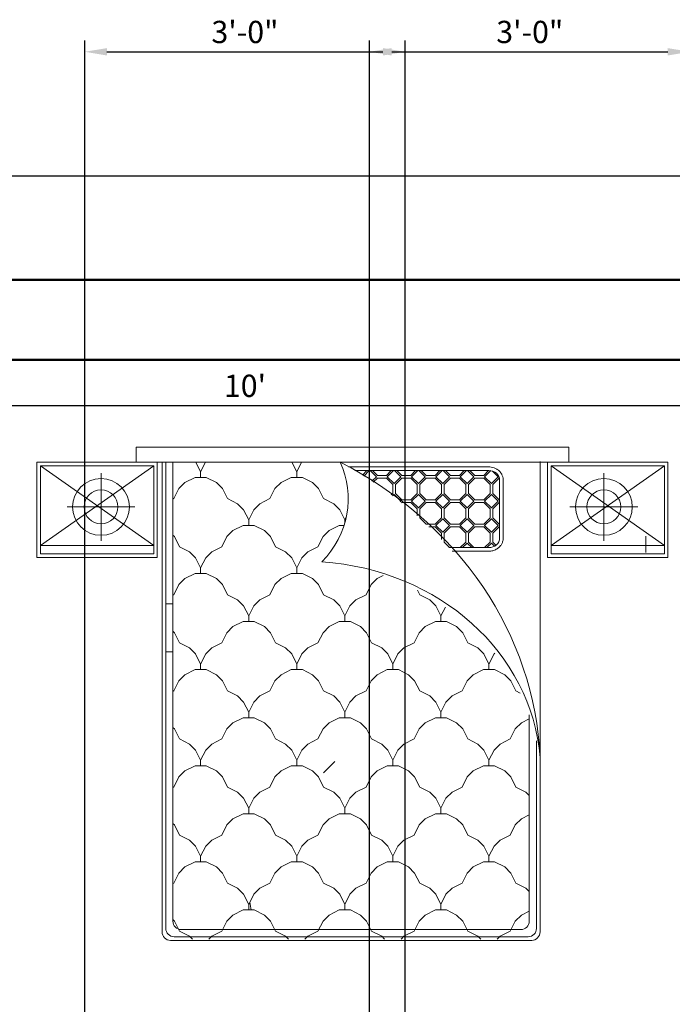
# Model space of a CAD drawing. Units: inches. Extents: x 2385 to 2740, y 1752 to 2305.
# Tile 14 of 15: x 2618 to 2691, y 2195 to 2305. Entities that reach past the tile are written whole.
import ezdxf

# ---------------------------------------------------------------- set-up
doc = ezdxf.new("R2010")
doc.units = ezdxf.units.IN
for name, color, linetype, lineweight in [('A-ANNO-DIMS', 2, 'Continuous', 18), ('A-FURN', 9, 'Continuous', 18), ('A-WALL', 7, 'Continuous', 50)]:
    doc.layers.add(name, color=color, linetype=linetype, lineweight=lineweight)
doc.styles.get("Standard").update_dxf_attribs({"font": 'arial.ttf'})
doc.dimstyles.new('Copy of ISO-25', dxfattribs={"dimtxt": 2.5, "dimasz": 2.5, "dimexe": 1.25, "dimexo": 0.625, "dimtad": 1, "dimdec": 1, "dimlunit": 4, "dimtxsty": 'Standard', "dimcen": 2.5, "dimadec": 0, "dimazin": 0, "dimtfac": 1, "dimtdec": 1, "dimtmove": 0, "dimatfit": 3, "dimfxl": 1, "dimarcsym": 0})

# ---------------------------------------------------------------- blocks, each defined once
blk = doc.blocks.new('A$C029D5C69')
for p, q in [((0.4164, 2.0693), (0.4164, 2.0066)), ((2.2315, 2.0693), (0.4164, 2.0693)), ((2.2315, 2.0066), (2.2315, 2.0693)), ((0, 1.606), (0, 2.0066)), ((0, 2.0066), (0.505, 2.0066)), ((0.0151, 1.6211), (0.0151, 1.9915)), ((0.0151, 1.9915), (0.4899, 1.9915)), ((0.4164, 2.0066), (2.2315, 2.0066)), ((0.4899, 1.9915), (0.4899, 1.6211)), ((0.505, 2.0066), (0.505, 1.606)), ((0.5252, 0.0351), (0.5252, 2.0066)), ((0.5403, 0.0502), (0.5403, 2.0066)), ((0.5706, 0.0805), (0.5706, 2.0066)), ((0.6869, 1.966), (0.6666, 2.0066)), ((0.7072, 2.0066), (0.6869, 1.966)), ((1.0902, 1.966), (1.0699, 2.0066)), ((1.1106, 2.0066), (1.0902, 1.966)), ((1.8954, 1.9865), (1.3081, 1.9865)), ((2.1114, 2.0087), (2.1114, 0.0351)), ((2.6479, 2.0066), (2.1429, 2.0066)), ((2.1429, 2.0066), (2.1429, 1.606)), ((2.6328, 1.9915), (2.158, 1.9915)), ((2.158, 1.9915), (2.158, 1.6211)), ((2.6328, 1.6211), (2.6328, 1.9915)), ((2.6479, 1.606), (2.6479, 2.0066)), ((0.2689, 1.9609), (0.2689, 1.6764)), ((0.6634, 1.9425), (0.621, 1.9213)), ((0.6634, 1.9425), (0.621, 1.9213)), ((0.6869, 1.9425), (0.6634, 1.9425)), ((0.6869, 1.9425), (0.6869, 1.966)), ((0.6869, 1.9425), (0.6869, 1.966)), ((0.6869, 1.9425), (0.7104, 1.9425)), ((0.7528, 1.9213), (0.7104, 1.9425)), ((0.7528, 1.9213), (0.7104, 1.9425)), ((1.0668, 1.9425), (1.0244, 1.9213)), ((1.0668, 1.9425), (1.0244, 1.9213)), ((1.0902, 1.9425), (1.0668, 1.9425)), ((1.0902, 1.9425), (1.0902, 1.966)), ((1.0902, 1.9425), (1.0902, 1.966)), ((1.0902, 1.9425), (1.1137, 1.9425)), ((1.1561, 1.9213), (1.1137, 1.9425)), ((1.1561, 1.9213), (1.1137, 1.9425)), ((1.8954, 1.9713), (1.3339, 1.9713)), ((1.3849, 1.9713), (1.3656, 1.952)), ((1.3945, 1.9713), (1.3714, 1.9483)), ((1.4249, 1.945), (1.3986, 1.9713)), ((1.4249, 1.945), (1.4059, 1.926)), ((1.4288, 1.9507), (1.4081, 1.9713)), ((1.4476, 1.9507), (1.4288, 1.9507)), ((1.4476, 1.9507), (1.4664, 1.9507)), ((1.487, 1.9713), (1.4664, 1.9507)), ((1.4966, 1.9713), (1.4703, 1.945)), ((1.4986, 1.9167), (1.4703, 1.945)), ((1.527, 1.945), (1.4986, 1.9167)), ((1.527, 1.945), (1.5007, 1.9713)), ((1.5309, 1.9507), (1.5102, 1.9713)), ((1.5497, 1.9507), (1.5309, 1.9507)), ((1.5497, 1.9507), (1.5685, 1.9507)), ((1.5891, 1.9713), (1.5685, 1.9507)), ((1.5987, 1.9713), (1.5724, 1.945)), ((1.6007, 1.9167), (1.5724, 1.945)), ((1.6291, 1.945), (1.6007, 1.9167)), ((1.6291, 1.945), (1.6028, 1.9713)), ((1.633, 1.9507), (1.6123, 1.9713)), ((1.6518, 1.9507), (1.633, 1.9507)), ((1.6518, 1.9507), (1.6706, 1.9507)), ((1.6912, 1.9713), (1.6706, 1.9507)), ((1.7008, 1.9713), (1.6745, 1.945)), ((1.7028, 1.9167), (1.6745, 1.945)), ((1.7312, 1.945), (1.7028, 1.9167)), ((1.7312, 1.945), (1.7049, 1.9713)), ((1.7351, 1.9507), (1.7144, 1.9713)), ((1.7539, 1.9507), (1.7351, 1.9507)), ((1.7539, 1.9507), (1.7727, 1.9507)), ((1.7933, 1.9713), (1.7727, 1.9507)), ((1.8029, 1.9713), (1.7766, 1.945)), ((1.8049, 1.9167), (1.7766, 1.945)), ((1.8333, 1.945), (1.8049, 1.9167)), ((1.8333, 1.945), (1.807, 1.9713)), ((1.8372, 1.9507), (1.8165, 1.9713)), ((1.856, 1.9507), (1.8372, 1.9507)), ((1.856, 1.9507), (1.8748, 1.9507)), ((1.8954, 1.9713), (1.8748, 1.9507)), ((1.9043, 1.9707), (1.8787, 1.945)), ((1.907, 1.9167), (1.8787, 1.945)), ((1.9354, 1.945), (1.907, 1.9167)), ((1.9354, 1.945), (1.9114, 1.969)), ((2.379, 1.9609), (2.379, 1.6764)), ((0.621, 1.9213), (0.5955, 1.8958)), ((0.7783, 1.8958), (0.7528, 1.9213)), ((1.0243, 1.9213), (0.9988, 1.8958)), ((1.1816, 1.8958), (1.1561, 1.9213)), ((1.4288, 1.9394), (1.4116, 1.9222)), ((1.4288, 1.9393), (1.4476, 1.9393)), ((1.4664, 1.9393), (1.4476, 1.9393)), ((1.493, 1.9128), (1.4664, 1.9394)), ((1.493, 1.8752), (1.493, 1.9128)), ((1.5309, 1.9394), (1.5043, 1.9128)), ((1.5043, 1.8752), (1.5043, 1.9128)), ((1.5309, 1.9393), (1.5497, 1.9393)), ((1.5685, 1.9393), (1.5497, 1.9393)), ((1.595, 1.9128), (1.5685, 1.9394)), ((1.595, 1.8752), (1.595, 1.9128)), ((1.633, 1.9394), (1.6064, 1.9128)), ((1.6064, 1.8752), (1.6064, 1.9128)), ((1.633, 1.9393), (1.6518, 1.9393)), ((1.6706, 1.9393), (1.6518, 1.9393)), ((1.6971, 1.9128), (1.6706, 1.9394)), ((1.6971, 1.8752), (1.6971, 1.9128)), ((1.7351, 1.9394), (1.7085, 1.9128)), ((1.7085, 1.8752), (1.7085, 1.9128)), ((1.7351, 1.9393), (1.7539, 1.9393)), ((1.7727, 1.9393), (1.7539, 1.9393)), ((1.7992, 1.9128), (1.7727, 1.9394)), ((1.7992, 1.8752), (1.7992, 1.9128)), ((1.8372, 1.9394), (1.8106, 1.9128)), ((1.8106, 1.8752), (1.8106, 1.9128)), ((1.8372, 1.9393), (1.856, 1.9393)), ((1.8748, 1.9393), (1.856, 1.9393)), ((1.9013, 1.9128), (1.8748, 1.9394)), ((1.9013, 1.8752), (1.9013, 1.9128)), ((1.9393, 1.9394), (1.9127, 1.9128)), ((1.9127, 1.8752), (1.9127, 1.9128)), ((1.9393, 1.9393), (1.9404, 1.9393)), ((1.9414, 1.688), (1.9414, 1.931)), ((1.9565, 1.688), (1.9565, 1.931)), ((0.5955, 1.8958), (0.5743, 1.8534)), ((0.7995, 1.8534), (0.7783, 1.8958)), ((0.9989, 1.8958), (0.9777, 1.8534)), ((1.2028, 1.8534), (1.1816, 1.8958)), ((1.493, 1.8752), (1.4867, 1.869)), ((1.4986, 1.8713), (1.4922, 1.8648)), ((1.527, 1.8429), (1.4986, 1.8713)), ((1.5309, 1.8486), (1.5043, 1.8752)), ((1.595, 1.8752), (1.5685, 1.8486)), ((1.6007, 1.8713), (1.5724, 1.8429)), ((1.6291, 1.8429), (1.6007, 1.8713)), ((1.633, 1.8486), (1.6064, 1.8752)), ((1.6971, 1.8752), (1.6706, 1.8486)), ((1.7028, 1.8713), (1.6745, 1.8429)), ((1.7312, 1.8429), (1.7028, 1.8713)), ((1.7351, 1.8486), (1.7085, 1.8752)), ((1.7992, 1.8752), (1.7727, 1.8486)), ((1.8049, 1.8713), (1.7766, 1.8429)), ((1.8333, 1.8429), (1.8049, 1.8713)), ((1.8372, 1.8486), (1.8106, 1.8752)), ((1.9013, 1.8752), (1.8748, 1.8486)), ((1.907, 1.8713), (1.8787, 1.8429)), ((1.9354, 1.8429), (1.907, 1.8713)), ((1.9393, 1.8486), (1.9127, 1.8752)), ((0.1267, 1.8186), (0.4111, 1.8186)), ((0.5743, 1.8534), (0.5706, 1.8515)), ((0.5743, 1.8534), (0.5706, 1.8515)), ((0.8419, 1.8322), (0.7995, 1.8534)), ((0.8419, 1.8322), (0.7995, 1.8534)), ((0.8674, 1.8067), (0.8419, 1.8322)), ((0.9352, 1.8322), (0.9097, 1.8067)), ((0.9777, 1.8534), (0.9353, 1.8322)), ((0.9777, 1.8534), (0.9353, 1.8322)), ((1.2452, 1.8322), (1.2028, 1.8534)), ((1.2452, 1.8322), (1.2028, 1.8534)), ((1.2707, 1.8067), (1.2452, 1.8322)), ((1.527, 1.8429), (1.5242, 1.8401)), ((1.5309, 1.8373), (1.5295, 1.8359)), ((1.5497, 1.8486), (1.5309, 1.8486)), ((1.5309, 1.8373), (1.5497, 1.8373)), ((1.5497, 1.8486), (1.5685, 1.8486)), ((1.5685, 1.8373), (1.5497, 1.8373)), ((1.595, 1.8107), (1.5685, 1.8373)), ((1.6007, 1.8146), (1.5724, 1.8429)), ((1.6291, 1.8429), (1.6007, 1.8146)), ((1.633, 1.8373), (1.6064, 1.8107)), ((1.6518, 1.8486), (1.633, 1.8486)), ((1.633, 1.8373), (1.6518, 1.8373)), ((1.6518, 1.8486), (1.6706, 1.8486)), ((1.6706, 1.8373), (1.6518, 1.8373)), ((1.6971, 1.8107), (1.6706, 1.8373)), ((1.7028, 1.8146), (1.6745, 1.8429)), ((1.7312, 1.8429), (1.7028, 1.8146)), ((1.7351, 1.8373), (1.7085, 1.8107)), ((1.7539, 1.8486), (1.7351, 1.8486)), ((1.7351, 1.8373), (1.7539, 1.8373)), ((1.7539, 1.8486), (1.7727, 1.8486)), ((1.7727, 1.8373), (1.7539, 1.8373)), ((1.7992, 1.8107), (1.7727, 1.8373)), ((1.8049, 1.8146), (1.7766, 1.8429)), ((1.8333, 1.8429), (1.8049, 1.8146)), ((1.8372, 1.8373), (1.8106, 1.8107)), ((1.856, 1.8486), (1.8372, 1.8486)), ((1.8372, 1.8373), (1.856, 1.8373)), ((1.856, 1.8486), (1.8748, 1.8486)), ((1.8748, 1.8373), (1.856, 1.8373)), ((1.9013, 1.8107), (1.8748, 1.8373)), ((1.907, 1.8146), (1.8787, 1.8429)), ((1.9354, 1.8429), (1.907, 1.8146)), ((1.9393, 1.8373), (1.9127, 1.8107)), ((1.9414, 1.8486), (1.9393, 1.8486)), ((1.9393, 1.8373), (1.9414, 1.8373)), ((2.2367, 1.8186), (2.5212, 1.8186)), ((0.8886, 1.7643), (0.8674, 1.8067)), ((0.9098, 1.8067), (0.8886, 1.7643)), ((1.2919, 1.7643), (1.2707, 1.8067)), ((1.2981, 1.7768), (1.2919, 1.7643)), ((1.595, 1.7806), (1.595, 1.8107)), ((1.6064, 1.7731), (1.6064, 1.8107)), ((1.6971, 1.7731), (1.6971, 1.8107)), ((1.7085, 1.7731), (1.7085, 1.8107)), ((1.7992, 1.7731), (1.7992, 1.8107)), ((1.8106, 1.7731), (1.8106, 1.8107)), ((1.9013, 1.7731), (1.9013, 1.8107)), ((1.9127, 1.7731), (1.9127, 1.8107)), ((0.8651, 1.7408), (0.8227, 1.7196)), ((0.8651, 1.7408), (0.8227, 1.7196)), ((0.912, 1.7408), (0.8651, 1.7408)), ((0.8886, 1.7408), (0.8886, 1.7643)), ((0.9544, 1.7196), (0.912, 1.7408)), ((0.9544, 1.7196), (0.912, 1.7408)), ((1.2684, 1.7408), (1.226, 1.7196)), ((1.2684, 1.7408), (1.226, 1.7196)), ((1.2885, 1.7408), (1.2684, 1.7408)), ((1.2919, 1.7519), (1.2919, 1.7643)), ((1.633, 1.7465), (1.6064, 1.7731)), ((1.6518, 1.7465), (1.633, 1.7465)), ((1.6443, 1.7352), (1.6518, 1.7352)), ((1.6518, 1.7465), (1.6706, 1.7465)), ((1.6706, 1.7352), (1.6518, 1.7352)), ((1.6971, 1.7731), (1.6706, 1.7465)), ((1.6971, 1.7086), (1.6706, 1.7352)), ((1.7028, 1.7692), (1.6745, 1.7408)), ((1.7028, 1.7125), (1.6745, 1.7408)), ((1.7312, 1.7408), (1.7028, 1.7692)), ((1.7312, 1.7408), (1.7028, 1.7125)), ((1.7351, 1.7465), (1.7085, 1.7731)), ((1.7351, 1.7352), (1.7085, 1.7086)), ((1.7539, 1.7465), (1.7351, 1.7465)), ((1.7351, 1.7352), (1.7539, 1.7352)), ((1.7539, 1.7465), (1.7727, 1.7465)), ((1.7727, 1.7352), (1.7539, 1.7352)), ((1.7992, 1.7731), (1.7727, 1.7465)), ((1.7992, 1.7086), (1.7727, 1.7352)), ((1.8049, 1.7692), (1.7766, 1.7408)), ((1.8049, 1.7125), (1.7766, 1.7408)), ((1.8333, 1.7408), (1.8049, 1.7692)), ((1.8333, 1.7408), (1.8049, 1.7125)), ((1.8372, 1.7465), (1.8106, 1.7731)), ((1.8372, 1.7352), (1.8106, 1.7086)), ((1.856, 1.7465), (1.8372, 1.7465)), ((1.8372, 1.7352), (1.856, 1.7352)), ((1.856, 1.7465), (1.8748, 1.7465)), ((1.8748, 1.7352), (1.856, 1.7352)), ((1.9013, 1.7731), (1.8748, 1.7465)), ((1.9013, 1.7086), (1.8748, 1.7352)), ((1.907, 1.7692), (1.8787, 1.7408)), ((1.907, 1.7125), (1.8787, 1.7408)), ((1.9354, 1.7408), (1.907, 1.7692)), ((1.9354, 1.7408), (1.907, 1.7125)), ((1.9393, 1.7465), (1.9127, 1.7731)), ((1.9393, 1.7352), (1.9127, 1.7086)), ((1.9414, 1.7465), (1.9393, 1.7465)), ((1.9393, 1.7352), (1.9414, 1.7352)), ((0.5766, 1.6941), (0.5706, 1.7002)), ((0.5978, 1.6517), (0.5766, 1.6941)), ((0.7972, 1.6941), (0.776, 1.6517)), ((0.8227, 1.7196), (0.7972, 1.6941)), ((0.98, 1.6941), (0.9545, 1.7196)), ((1.0011, 1.6517), (0.9799, 1.6941)), ((1.2005, 1.6941), (1.1793, 1.6517)), ((1.226, 1.7196), (1.2005, 1.6941)), ((1.6971, 1.682), (1.6971, 1.7086)), ((1.7085, 1.671), (1.7085, 1.7086)), ((1.7992, 1.671), (1.7992, 1.7086)), ((1.8106, 1.671), (1.8106, 1.7086)), ((1.9013, 1.671), (1.9013, 1.7086)), ((1.9127, 1.671), (1.9127, 1.7086)), ((2.5551, 1.6275), (2.5551, 1.696)), ((1.7318, 1.6477), (1.7085, 1.671)), ((1.7992, 1.671), (1.7759, 1.6477)), ((1.8049, 1.6671), (1.7855, 1.6477)), ((1.8244, 1.6477), (1.8049, 1.6671)), ((1.8339, 1.6477), (1.8106, 1.671)), ((1.9013, 1.671), (1.878, 1.6477)), ((1.907, 1.6671), (1.8876, 1.6477)), ((1.9202, 1.6539), (1.907, 1.6671)), ((1.926, 1.6577), (1.9127, 1.671)), ((0.4899, 1.6211), (0.0151, 1.6211)), ((0.6402, 1.6305), (0.5978, 1.6517)), ((0.6402, 1.6305), (0.5978, 1.6517)), ((0.6657, 1.605), (0.6402, 1.6305)), ((0.7336, 1.6305), (0.7081, 1.605)), ((0.776, 1.6517), (0.7336, 1.6305)), ((0.776, 1.6517), (0.7336, 1.6305)), ((1.0435, 1.6305), (1.0011, 1.6517)), ((1.0435, 1.6305), (1.0011, 1.6517)), ((1.0691, 1.605), (1.0436, 1.6305)), ((1.1369, 1.6305), (1.1114, 1.605)), ((1.1793, 1.6517), (1.1369, 1.6305)), ((1.1793, 1.6517), (1.1369, 1.6305)), ((1.8961, 1.6477), (1.7289, 1.6477)), ((1.8961, 1.6325), (1.7422, 1.6325)), ((2.158, 1.6211), (2.6328, 1.6211)), ((0.505, 1.606), (0, 1.606)), ((0.6869, 1.5626), (0.6657, 1.605)), ((0.7081, 1.605), (0.6869, 1.5626)), ((1.0902, 1.5626), (1.069, 1.605)), ((1.1114, 1.605), (1.0902, 1.5626)), ((2.1429, 1.606), (2.6479, 1.606)), ((0.6634, 1.5391), (0.621, 1.5179)), ((0.6634, 1.5391), (0.621, 1.5179)), ((0.6869, 1.5392), (0.6634, 1.5392)), ((0.6869, 1.5392), (0.6869, 1.5626)), ((0.6869, 1.5392), (0.6869, 1.5626)), ((0.6869, 1.5392), (0.7104, 1.5392)), ((0.7528, 1.5179), (0.7104, 1.5391)), ((0.7528, 1.5179), (0.7104, 1.5391)), ((1.0668, 1.5391), (1.0244, 1.5179)), ((1.0668, 1.5391), (1.0244, 1.5179)), ((1.0902, 1.5392), (1.0668, 1.5392)), ((1.0902, 1.5392), (1.0902, 1.5626)), ((1.0902, 1.5392), (1.0902, 1.5626)), ((1.0902, 1.5392), (1.1137, 1.5392)), ((1.1561, 1.5179), (1.1137, 1.5391)), ((1.1561, 1.5179), (1.1137, 1.5391)), ((1.4534, 1.5308), (1.4277, 1.5179)), ((1.4534, 1.5308), (1.4277, 1.5179)), ((0.5955, 1.4925), (0.5743, 1.4501)), ((0.621, 1.5179), (0.5955, 1.4924)), ((0.7783, 1.4924), (0.7528, 1.5179)), ((0.7995, 1.4501), (0.7783, 1.4925)), ((0.9989, 1.4925), (0.9777, 1.4501)), ((1.0243, 1.5179), (0.9988, 1.4924)), ((1.1816, 1.4924), (1.1561, 1.5179)), ((1.2028, 1.4501), (1.1816, 1.4925)), ((1.4022, 1.4925), (1.381, 1.4501)), ((1.4277, 1.5179), (1.4022, 1.4924)), ((0.5743, 1.45), (0.5706, 1.4481)), ((0.5743, 1.45), (0.5706, 1.4481)), ((0.8419, 1.4288), (0.7995, 1.45)), ((0.8419, 1.4288), (0.7995, 1.45)), ((0.9777, 1.45), (0.9353, 1.4288)), ((0.9777, 1.45), (0.9353, 1.4288)), ((1.2452, 1.4288), (1.2028, 1.45)), ((1.2452, 1.4288), (1.2028, 1.45)), ((1.381, 1.45), (1.3386, 1.4288)), ((1.381, 1.45), (1.3386, 1.4288)), ((1.6062, 1.4501), (1.5966, 1.4692)), ((1.6486, 1.4288), (1.6062, 1.45)), ((1.6486, 1.4288), (1.6062, 1.45)), ((0.5403, 1.4117), (0.5706, 1.4117)), ((0.8674, 1.4033), (0.8419, 1.4288)), ((0.9352, 1.4288), (0.9097, 1.4033)), ((1.2707, 1.4033), (1.2452, 1.4288)), ((1.3386, 1.4288), (1.3131, 1.4033)), ((1.6741, 1.4033), (1.6486, 1.4288)), ((0.8886, 1.361), (0.8674, 1.4034)), ((0.9098, 1.4034), (0.8886, 1.361)), ((1.2919, 1.361), (1.2707, 1.4034)), ((1.3131, 1.4034), (1.2919, 1.361)), ((1.6953, 1.361), (1.6741, 1.4034)), ((1.714, 1.3984), (1.6953, 1.361)), ((0.8651, 1.3374), (0.8227, 1.3162)), ((0.8651, 1.3374), (0.8227, 1.3162)), ((0.912, 1.3375), (0.8651, 1.3375)), ((0.8886, 1.3375), (0.8886, 1.3609)), ((0.9544, 1.3162), (0.912, 1.3374)), ((0.9544, 1.3162), (0.912, 1.3374)), ((1.2684, 1.3374), (1.226, 1.3162)), ((1.2684, 1.3374), (1.226, 1.3162)), ((1.3154, 1.3375), (1.2684, 1.3375)), ((1.2919, 1.3375), (1.2919, 1.3609)), ((1.3578, 1.3162), (1.3154, 1.3374)), ((1.3578, 1.3162), (1.3154, 1.3374)), ((1.6718, 1.3374), (1.6294, 1.3162)), ((1.6718, 1.3374), (1.6294, 1.3162)), ((1.7187, 1.3375), (1.6718, 1.3375)), ((1.6953, 1.3375), (1.6953, 1.3609)), ((1.7611, 1.3162), (1.7187, 1.3374)), ((1.7611, 1.3162), (1.7187, 1.3374)), ((0.5766, 1.2908), (0.5706, 1.2968)), ((0.5978, 1.2484), (0.5766, 1.2908)), ((0.7972, 1.2908), (0.776, 1.2484)), ((0.8227, 1.3163), (0.7972, 1.2908)), ((0.98, 1.2908), (0.9545, 1.3163)), ((1.0011, 1.2484), (0.9799, 1.2908)), ((1.2005, 1.2908), (1.1793, 1.2484)), ((1.226, 1.3163), (1.2005, 1.2908)), ((1.3833, 1.2908), (1.3578, 1.3163)), ((1.4045, 1.2484), (1.3833, 1.2908)), ((1.6039, 1.2908), (1.5827, 1.2484)), ((1.6294, 1.3163), (1.6039, 1.2908)), ((1.7867, 1.2908), (1.7611, 1.3163)), ((1.8078, 1.2484), (1.7866, 1.2908)), ((0.6402, 1.2271), (0.5978, 1.2483)), ((0.6402, 1.2271), (0.5978, 1.2483)), ((0.776, 1.2483), (0.7336, 1.2271)), ((0.776, 1.2483), (0.7336, 1.2271)), ((1.0435, 1.2271), (1.0011, 1.2483)), ((1.0435, 1.2271), (1.0011, 1.2483)), ((1.1793, 1.2483), (1.1369, 1.2271)), ((1.1793, 1.2483), (1.1369, 1.2271)), ((1.4469, 1.2271), (1.4045, 1.2483)), ((1.4469, 1.2271), (1.4045, 1.2483)), ((1.5827, 1.2483), (1.5403, 1.2271)), ((1.5827, 1.2483), (1.5403, 1.2271)), ((1.8502, 1.2271), (1.8078, 1.2483)), ((1.8502, 1.2271), (1.8078, 1.2483)), ((0.5403, 1.21), (0.5706, 1.21)), ((0.6657, 1.2017), (0.6402, 1.2272)), ((0.6869, 1.1593), (0.6657, 1.2017)), ((0.7081, 1.2017), (0.6869, 1.1593)), ((0.7336, 1.2272), (0.7081, 1.2017)), ((1.0691, 1.2017), (1.0436, 1.2272)), ((1.0902, 1.1593), (1.069, 1.2017)), ((1.1114, 1.2017), (1.0902, 1.1593)), ((1.1369, 1.2272), (1.1114, 1.2017)), ((1.4724, 1.2017), (1.4469, 1.2272)), ((1.4936, 1.1593), (1.4724, 1.2017)), ((1.5148, 1.2017), (1.4936, 1.1593)), ((1.5403, 1.2272), (1.5148, 1.2017)), ((1.8758, 1.2017), (1.8503, 1.2272)), ((1.8969, 1.1593), (1.8757, 1.2017)), ((1.9181, 1.2017), (1.8969, 1.1593)), ((1.9215, 1.2051), (1.9181, 1.2017)), ((0.6869, 1.1358), (0.6869, 1.1593)), ((0.6869, 1.1358), (0.6869, 1.1593)), ((1.0902, 1.1358), (1.0902, 1.1593)), ((1.0902, 1.1358), (1.0902, 1.1593)), ((1.4936, 1.1358), (1.4936, 1.1593)), ((1.4936, 1.1358), (1.4936, 1.1593)), ((1.8969, 1.1358), (1.8969, 1.1593)), ((1.8969, 1.1358), (1.8969, 1.1593)), ((0.6634, 1.1358), (0.621, 1.1146)), ((0.6634, 1.1358), (0.621, 1.1146)), ((0.6869, 1.1358), (0.6634, 1.1358)), ((0.6869, 1.1358), (0.7104, 1.1358)), ((0.7528, 1.1146), (0.7104, 1.1358)), ((0.7528, 1.1146), (0.7104, 1.1358)), ((1.0668, 1.1358), (1.0244, 1.1146)), ((1.0668, 1.1358), (1.0244, 1.1146)), ((1.0902, 1.1358), (1.0668, 1.1358)), ((1.0902, 1.1358), (1.1137, 1.1358)), ((1.1561, 1.1146), (1.1137, 1.1358)), ((1.1561, 1.1146), (1.1137, 1.1358)), ((1.4701, 1.1358), (1.4277, 1.1146)), ((1.4701, 1.1358), (1.4277, 1.1146)), ((1.4936, 1.1358), (1.4701, 1.1358)), ((1.4936, 1.1358), (1.5171, 1.1358)), ((1.5595, 1.1146), (1.5171, 1.1358)), ((1.5595, 1.1146), (1.5171, 1.1358)), ((1.8735, 1.1358), (1.8311, 1.1146)), ((1.8735, 1.1358), (1.8311, 1.1146)), ((1.8969, 1.1358), (1.8735, 1.1358)), ((1.8969, 1.1358), (1.9204, 1.1358)), ((1.9628, 1.1146), (1.9204, 1.1358)), ((1.9628, 1.1146), (1.9204, 1.1358)), ((0.5955, 1.0891), (0.5743, 1.0467)), ((0.621, 1.1146), (0.5955, 1.0891)), ((0.7783, 1.0891), (0.7528, 1.1146)), ((0.7995, 1.0467), (0.7783, 1.0891)), ((0.9989, 1.0891), (0.9777, 1.0467)), ((1.0243, 1.1146), (0.9988, 1.0891)), ((1.1816, 1.0891), (1.1561, 1.1146)), ((1.2028, 1.0467), (1.1816, 1.0891)), ((1.4022, 1.0891), (1.381, 1.0467)), ((1.4277, 1.1146), (1.4022, 1.0891)), ((1.585, 1.0891), (1.5595, 1.1146)), ((1.6062, 1.0467), (1.585, 1.0891)), ((1.8056, 1.0891), (1.7844, 1.0467)), ((1.831, 1.1146), (1.8055, 1.0891)), ((1.9883, 1.0891), (1.9628, 1.1146)), ((2.0095, 1.0467), (1.9883, 1.0891)), ((0.5743, 1.0467), (0.5706, 1.0448)), ((0.5743, 1.0467), (0.5706, 1.0448)), ((0.8419, 1.0255), (0.7995, 1.0467)), ((0.8419, 1.0255), (0.7995, 1.0467)), ((0.9777, 1.0467), (0.9353, 1.0255)), ((0.9777, 1.0467), (0.9353, 1.0255)), ((1.2452, 1.0255), (1.2028, 1.0467)), ((1.2452, 1.0255), (1.2028, 1.0467)), ((1.381, 1.0467), (1.3386, 1.0255)), ((1.381, 1.0467), (1.3386, 1.0255)), ((1.6486, 1.0255), (1.6062, 1.0467)), ((1.6486, 1.0255), (1.6062, 1.0467)), ((1.7844, 1.0467), (1.742, 1.0255)), ((1.7844, 1.0467), (1.742, 1.0255)), ((2.0276, 1.0376), (2.0095, 1.0467)), ((2.0276, 1.0376), (2.0095, 1.0467)), ((0.8674, 1), (0.8419, 1.0255)), ((0.8886, 0.9576), (0.8674, 1)), ((0.9098, 1), (0.8886, 0.9576)), ((0.9352, 1.0255), (0.9097, 1)), ((1.2707, 1), (1.2452, 1.0255)), ((1.2919, 0.9576), (1.2707, 1)), ((1.3131, 1), (1.2919, 0.9576)), ((1.3386, 1.0255), (1.3131, 1)), ((1.6741, 1), (1.6486, 1.0255)), ((1.6953, 0.9576), (1.6741, 1)), ((1.7165, 1), (1.6953, 0.9576)), ((1.7419, 1.0255), (1.7164, 1)), ((0.8886, 0.9341), (0.8886, 0.9576)), ((1.2919, 0.9341), (1.2919, 0.9576)), ((1.6953, 0.9341), (1.6953, 0.9576)), ((0.8227, 0.9129), (0.7972, 0.8874)), ((0.8651, 0.9341), (0.8227, 0.9129)), ((0.8651, 0.9341), (0.8227, 0.9129)), ((0.912, 0.9341), (0.8651, 0.9341)), ((0.9544, 0.9129), (0.912, 0.9341)), ((0.9544, 0.9129), (0.912, 0.9341)), ((0.98, 0.8874), (0.9545, 0.9129)), ((1.226, 0.9129), (1.2005, 0.8874)), ((1.2684, 0.9341), (1.226, 0.9129)), ((1.2684, 0.9341), (1.226, 0.9129)), ((1.3154, 0.9341), (1.2684, 0.9341)), ((1.3578, 0.9129), (1.3154, 0.9341)), ((1.3578, 0.9129), (1.3154, 0.9341)), ((1.3833, 0.8874), (1.3578, 0.9129)), ((1.6294, 0.9129), (1.6039, 0.8874)), ((1.6718, 0.9341), (1.6294, 0.9129)), ((1.6718, 0.9341), (1.6294, 0.9129)), ((1.7187, 0.9341), (1.6718, 0.9341)), ((1.7611, 0.9129), (1.7187, 0.9341)), ((1.7611, 0.9129), (1.7187, 0.9341)), ((1.7867, 0.8874), (1.7611, 0.9129)), ((2.0327, 0.9129), (2.0072, 0.8874)), ((2.066, 0.9295), (2.0327, 0.9129)), ((2.066, 0.9295), (2.0327, 0.9129)), ((2.066, 0.9457), (2.066, 0.0805)), ((0.5766, 0.8874), (0.5706, 0.8935)), ((0.5978, 0.845), (0.5766, 0.8874)), ((0.7972, 0.8874), (0.776, 0.845)), ((1.0011, 0.845), (0.9799, 0.8874)), ((1.2005, 0.8874), (1.1793, 0.845)), ((1.4045, 0.845), (1.3833, 0.8874)), ((1.6039, 0.8874), (1.5827, 0.845)), ((1.8078, 0.845), (1.7866, 0.8874)), ((2.0072, 0.8874), (1.986, 0.845)), ((0.6402, 0.8238), (0.5978, 0.845)), ((0.6402, 0.8238), (0.5978, 0.845)), ((0.776, 0.845), (0.7336, 0.8238)), ((0.776, 0.845), (0.7336, 0.8238)), ((1.0435, 0.8238), (1.0011, 0.845)), ((1.0435, 0.8238), (1.0011, 0.845)), ((1.1793, 0.845), (1.1369, 0.8238)), ((1.1793, 0.845), (1.1369, 0.8238)), ((1.4469, 0.8238), (1.4045, 0.845)), ((1.4469, 0.8238), (1.4045, 0.845)), ((1.5827, 0.845), (1.5403, 0.8238)), ((1.5827, 0.845), (1.5403, 0.8238)), ((1.8502, 0.8238), (1.8078, 0.845)), ((1.8502, 0.8238), (1.8078, 0.845)), ((1.986, 0.845), (1.9436, 0.8238)), ((1.986, 0.845), (1.9436, 0.8238)), ((2.0962, 0.8369), (2.0962, 0.0502)), ((0.6657, 0.7983), (0.6402, 0.8238)), ((0.6869, 0.7559), (0.6657, 0.7983)), ((0.7081, 0.7983), (0.6869, 0.7559)), ((0.7336, 0.8238), (0.7081, 0.7983)), ((1.0691, 0.7983), (1.0436, 0.8238)), ((1.0902, 0.7559), (1.069, 0.7983)), ((1.1114, 0.7983), (1.0902, 0.7559)), ((1.1369, 0.8238), (1.1114, 0.7983)), ((1.4724, 0.7983), (1.4469, 0.8238)), ((1.4936, 0.7559), (1.4724, 0.7983)), ((1.5148, 0.7983), (1.4936, 0.7559)), ((1.5403, 0.8238), (1.5148, 0.7983)), ((1.8758, 0.7983), (1.8503, 0.8238)), ((1.8969, 0.7559), (1.8757, 0.7983)), ((1.9181, 0.7983), (1.8969, 0.7559)), ((1.9436, 0.8238), (1.9181, 0.7983)), ((0.6869, 0.7325), (0.6869, 0.7559)), ((0.6869, 0.7325), (0.6869, 0.7559)), ((1.0902, 0.7325), (1.0902, 0.7559)), ((1.0902, 0.7325), (1.0902, 0.7559)), ((1.2024, 0.7028), (1.2503, 0.7507)), ((1.4936, 0.7325), (1.4936, 0.7559)), ((1.4936, 0.7325), (1.4936, 0.7559)), ((1.8969, 0.7325), (1.8969, 0.7559)), ((1.8969, 0.7325), (1.8969, 0.7559)), ((0.621, 0.7113), (0.5955, 0.6858)), ((0.6634, 0.7324), (0.621, 0.7112)), ((0.6634, 0.7324), (0.621, 0.7112)), ((0.6869, 0.7325), (0.6634, 0.7325)), ((0.6869, 0.7325), (0.7104, 0.7325)), ((0.7528, 0.7112), (0.7104, 0.7324)), ((0.7528, 0.7112), (0.7104, 0.7324)), ((0.7783, 0.6858), (0.7528, 0.7113)), ((1.0243, 0.7113), (0.9988, 0.6858)), ((1.0668, 0.7324), (1.0244, 0.7112)), ((1.0668, 0.7324), (1.0244, 0.7112)), ((1.0902, 0.7325), (1.0668, 0.7325)), ((1.0902, 0.7325), (1.1137, 0.7325)), ((1.1561, 0.7112), (1.1137, 0.7324)), ((1.1561, 0.7112), (1.1137, 0.7324)), ((1.1816, 0.6858), (1.1561, 0.7113)), ((1.4277, 0.7113), (1.4022, 0.6858)), ((1.4701, 0.7324), (1.4277, 0.7112)), ((1.4701, 0.7324), (1.4277, 0.7112)), ((1.4936, 0.7325), (1.4701, 0.7325)), ((1.4936, 0.7325), (1.5171, 0.7325)), ((1.5595, 0.7112), (1.5171, 0.7324)), ((1.5595, 0.7112), (1.5171, 0.7324)), ((1.585, 0.6858), (1.5595, 0.7113)), ((1.831, 0.7113), (1.8055, 0.6858)), ((1.8735, 0.7324), (1.8311, 0.7112)), ((1.8735, 0.7324), (1.8311, 0.7112)), ((1.8969, 0.7325), (1.8735, 0.7325)), ((1.8969, 0.7325), (1.9204, 0.7325)), ((1.9628, 0.7112), (1.9204, 0.7324)), ((1.9628, 0.7112), (1.9204, 0.7324)), ((1.9883, 0.6858), (1.9628, 0.7113)), ((0.5955, 0.6858), (0.5743, 0.6434)), ((0.7995, 0.6434), (0.7783, 0.6858)), ((0.9989, 0.6858), (0.9777, 0.6434)), ((1.2028, 0.6434), (1.1816, 0.6858)), ((1.4022, 0.6858), (1.381, 0.6434)), ((1.6062, 0.6434), (1.585, 0.6858)), ((1.8056, 0.6858), (1.7844, 0.6434)), ((2.0095, 0.6434), (1.9883, 0.6858)), ((0.5743, 0.6433), (0.5706, 0.6414)), ((0.5743, 0.6433), (0.5706, 0.6414)), ((0.8419, 0.6221), (0.7995, 0.6433)), ((0.8419, 0.6221), (0.7995, 0.6433)), ((0.8674, 0.5967), (0.8419, 0.6222)), ((0.9352, 0.6222), (0.9097, 0.5967)), ((0.9777, 0.6433), (0.9353, 0.6221)), ((0.9777, 0.6433), (0.9353, 0.6221)), ((1.2452, 0.6221), (1.2028, 0.6433)), ((1.2452, 0.6221), (1.2028, 0.6433)), ((1.2707, 0.5967), (1.2452, 0.6222)), ((1.3386, 0.6222), (1.3131, 0.5967)), ((1.381, 0.6433), (1.3386, 0.6221)), ((1.381, 0.6433), (1.3386, 0.6221)), ((1.6486, 0.6221), (1.6062, 0.6433)), ((1.6486, 0.6221), (1.6062, 0.6433)), ((1.6741, 0.5967), (1.6486, 0.6222)), ((1.7419, 0.6222), (1.7164, 0.5967)), ((1.7844, 0.6433), (1.742, 0.6221)), ((1.7844, 0.6433), (1.742, 0.6221)), ((2.0519, 0.6221), (2.0095, 0.6433)), ((2.0519, 0.6221), (2.0095, 0.6433)), ((2.066, 0.6081), (2.0519, 0.6222)), ((0.8886, 0.5543), (0.8674, 0.5967)), ((0.9098, 0.5967), (0.8886, 0.5543)), ((1.2919, 0.5543), (1.2707, 0.5967)), ((1.3131, 0.5967), (1.2919, 0.5543)), ((1.6953, 0.5543), (1.6741, 0.5967)), ((1.7165, 0.5967), (1.6953, 0.5543)), ((0.8886, 0.5308), (0.8886, 0.5543)), ((1.2919, 0.5308), (1.2919, 0.5543)), ((1.6953, 0.5308), (1.6953, 0.5543)), ((0.8227, 0.5096), (0.7972, 0.4841)), ((0.8651, 0.5308), (0.8227, 0.5096)), ((0.8651, 0.5308), (0.8227, 0.5096)), ((0.912, 0.5308), (0.8651, 0.5308)), ((0.9544, 0.5096), (0.912, 0.5308)), ((0.9544, 0.5096), (0.912, 0.5308)), ((0.98, 0.4841), (0.9545, 0.5096)), ((1.226, 0.5096), (1.2005, 0.4841)), ((1.2684, 0.5308), (1.226, 0.5096)), ((1.2684, 0.5308), (1.226, 0.5096)), ((1.3154, 0.5308), (1.2684, 0.5308)), ((1.3578, 0.5096), (1.3154, 0.5308)), ((1.3578, 0.5096), (1.3154, 0.5308)), ((1.3833, 0.4841), (1.3578, 0.5096)), ((1.6294, 0.5096), (1.6039, 0.4841)), ((1.6718, 0.5308), (1.6294, 0.5096)), ((1.6718, 0.5308), (1.6294, 0.5096)), ((1.7187, 0.5308), (1.6718, 0.5308)), ((1.7611, 0.5096), (1.7187, 0.5308)), ((1.7611, 0.5096), (1.7187, 0.5308)), ((1.7867, 0.4841), (1.7611, 0.5096)), ((2.0327, 0.5096), (2.0072, 0.4841)), ((2.066, 0.5262), (2.0327, 0.5096)), ((2.066, 0.5262), (2.0327, 0.5096)), ((0.5766, 0.4841), (0.5706, 0.4901)), ((0.5978, 0.4417), (0.5766, 0.4841)), ((0.7972, 0.4841), (0.776, 0.4417)), ((1.0011, 0.4417), (0.9799, 0.4841)), ((1.2005, 0.4841), (1.1793, 0.4417)), ((1.4045, 0.4417), (1.3833, 0.4841)), ((1.6039, 0.4841), (1.5827, 0.4417)), ((1.8078, 0.4417), (1.7866, 0.4841)), ((2.0072, 0.4841), (1.986, 0.4417)), ((0.6402, 0.4205), (0.5978, 0.4417)), ((0.6402, 0.4205), (0.5978, 0.4417)), ((0.6657, 0.395), (0.6402, 0.4205)), ((0.7336, 0.4205), (0.7081, 0.395)), ((0.776, 0.4417), (0.7336, 0.4205)), ((0.776, 0.4417), (0.7336, 0.4205)), ((1.0435, 0.4205), (1.0011, 0.4417)), ((1.0435, 0.4205), (1.0011, 0.4417)), ((1.0691, 0.395), (1.0436, 0.4205)), ((1.1369, 0.4205), (1.1114, 0.395)), ((1.1793, 0.4417), (1.1369, 0.4205)), ((1.1793, 0.4417), (1.1369, 0.4205)), ((1.4469, 0.4205), (1.4045, 0.4417)), ((1.4469, 0.4205), (1.4045, 0.4417)), ((1.4724, 0.395), (1.4469, 0.4205)), ((1.5403, 0.4205), (1.5148, 0.395)), ((1.5827, 0.4417), (1.5403, 0.4205)), ((1.5827, 0.4417), (1.5403, 0.4205)), ((1.8502, 0.4205), (1.8078, 0.4417)), ((1.8502, 0.4205), (1.8078, 0.4417)), ((1.8758, 0.395), (1.8503, 0.4205)), ((1.9436, 0.4205), (1.9181, 0.395)), ((1.986, 0.4417), (1.9436, 0.4205)), ((1.986, 0.4417), (1.9436, 0.4205)), ((0.6869, 0.3526), (0.6657, 0.395)), ((0.7081, 0.395), (0.6869, 0.3526)), ((1.0902, 0.3526), (1.069, 0.395)), ((1.1114, 0.395), (1.0902, 0.3526)), ((1.4936, 0.3526), (1.4724, 0.395)), ((1.5148, 0.395), (1.4936, 0.3526)), ((1.8969, 0.3526), (1.8757, 0.395)), ((1.9181, 0.395), (1.8969, 0.3526)), ((0.6869, 0.3291), (0.6869, 0.3526)), ((0.6869, 0.3291), (0.6869, 0.3526)), ((1.0902, 0.3291), (1.0902, 0.3526)), ((1.0902, 0.3291), (1.0902, 0.3526)), ((1.4936, 0.3291), (1.4936, 0.3526)), ((1.4936, 0.3291), (1.4936, 0.3526)), ((1.8969, 0.3291), (1.8969, 0.3526)), ((1.8969, 0.3291), (1.8969, 0.3526)), ((0.621, 0.3079), (0.5955, 0.2824)), ((0.6634, 0.3291), (0.621, 0.3079)), ((0.6634, 0.3291), (0.621, 0.3079)), ((0.6869, 0.3291), (0.6634, 0.3291)), ((0.6869, 0.3291), (0.7104, 0.3291)), ((0.7528, 0.3079), (0.7104, 0.3291)), ((0.7528, 0.3079), (0.7104, 0.3291)), ((0.7783, 0.2824), (0.7528, 0.3079)), ((1.0243, 0.3079), (0.9988, 0.2824)), ((1.0668, 0.3291), (1.0244, 0.3079)), ((1.0668, 0.3291), (1.0244, 0.3079)), ((1.0902, 0.3291), (1.0668, 0.3291)), ((1.0902, 0.3291), (1.1137, 0.3291)), ((1.1561, 0.3079), (1.1137, 0.3291)), ((1.1561, 0.3079), (1.1137, 0.3291)), ((1.1816, 0.2824), (1.1561, 0.3079)), ((1.4277, 0.3079), (1.4022, 0.2824)), ((1.4701, 0.3291), (1.4277, 0.3079)), ((1.4701, 0.3291), (1.4277, 0.3079)), ((1.4936, 0.3291), (1.4701, 0.3291)), ((1.4936, 0.3291), (1.5171, 0.3291)), ((1.5595, 0.3079), (1.5171, 0.3291)), ((1.5595, 0.3079), (1.5171, 0.3291)), ((1.585, 0.2824), (1.5595, 0.3079)), ((1.831, 0.3079), (1.8055, 0.2824)), ((1.8735, 0.3291), (1.8311, 0.3079)), ((1.8735, 0.3291), (1.8311, 0.3079)), ((1.8969, 0.3291), (1.8735, 0.3291)), ((1.8969, 0.3291), (1.9204, 0.3291)), ((1.9628, 0.3079), (1.9204, 0.3291)), ((1.9628, 0.3079), (1.9204, 0.3291)), ((1.9883, 0.2824), (1.9628, 0.3079)), ((0.5955, 0.2824), (0.5743, 0.24)), ((0.7995, 0.24), (0.7783, 0.2824)), ((0.9989, 0.2824), (0.9777, 0.24)), ((1.2028, 0.24), (1.1816, 0.2824)), ((1.4022, 0.2824), (1.381, 0.24)), ((1.6062, 0.24), (1.585, 0.2824)), ((1.8056, 0.2824), (1.7844, 0.24)), ((2.0095, 0.24), (1.9883, 0.2824)), ((0.5743, 0.24), (0.5706, 0.2381)), ((0.5743, 0.24), (0.5706, 0.2381)), ((0.8419, 0.2188), (0.7995, 0.24)), ((0.8419, 0.2188), (0.7995, 0.24)), ((0.8674, 0.1933), (0.8419, 0.2188)), ((0.9352, 0.2188), (0.9097, 0.1933)), ((0.9777, 0.24), (0.9353, 0.2188)), ((0.9777, 0.24), (0.9353, 0.2188)), ((1.2452, 0.2188), (1.2028, 0.24)), ((1.2452, 0.2188), (1.2028, 0.24)), ((1.2707, 0.1933), (1.2452, 0.2188)), ((1.3386, 0.2188), (1.3131, 0.1933)), ((1.381, 0.24), (1.3386, 0.2188)), ((1.381, 0.24), (1.3386, 0.2188)), ((1.6486, 0.2188), (1.6062, 0.24)), ((1.6486, 0.2188), (1.6062, 0.24)), ((1.6741, 0.1933), (1.6486, 0.2188)), ((1.7419, 0.2188), (1.7164, 0.1933)), ((1.7844, 0.24), (1.742, 0.2188)), ((1.7844, 0.24), (1.742, 0.2188)), ((2.0519, 0.2188), (2.0095, 0.24)), ((2.0519, 0.2188), (2.0095, 0.24)), ((2.066, 0.2047), (2.0519, 0.2188)), ((0.8886, 0.1509), (0.8674, 0.1933)), ((0.9098, 0.1933), (0.8886, 0.1509)), ((1.2919, 0.1509), (1.2707, 0.1933)), ((1.3131, 0.1933), (1.2919, 0.1509)), ((1.6953, 0.1509), (1.6741, 0.1933)), ((1.7165, 0.1933), (1.6953, 0.1509)), ((0.8651, 0.1274), (0.8227, 0.1062)), ((0.8651, 0.1274), (0.8227, 0.1062)), ((0.912, 0.1275), (0.8651, 0.1275)), ((0.8886, 0.1275), (0.8886, 0.1509)), ((0.9544, 0.1062), (0.912, 0.1274)), ((0.9544, 0.1062), (0.912, 0.1274)), ((1.2684, 0.1274), (1.226, 0.1062)), ((1.2684, 0.1274), (1.226, 0.1062)), ((1.3154, 0.1275), (1.2684, 0.1275)), ((1.2919, 0.1275), (1.2919, 0.1509)), ((1.3578, 0.1062), (1.3154, 0.1274)), ((1.3578, 0.1062), (1.3154, 0.1274)), ((1.6718, 0.1274), (1.6294, 0.1062)), ((1.6718, 0.1274), (1.6294, 0.1062)), ((1.7187, 0.1275), (1.6718, 0.1275)), ((1.6953, 0.1275), (1.6953, 0.1509)), ((1.7611, 0.1062), (1.7187, 0.1274)), ((1.7611, 0.1062), (1.7187, 0.1274)), ((0.5766, 0.0807), (0.5706, 0.0868)), ((0.8227, 0.1062), (0.7972, 0.0807)), ((0.98, 0.0807), (0.9545, 0.1062)), ((1.226, 0.1062), (1.2005, 0.0807)), ((1.3833, 0.0807), (1.3578, 0.1062)), ((1.6294, 0.1062), (1.6039, 0.0807)), ((1.7867, 0.0807), (1.7611, 0.1062)), ((2.0327, 0.1062), (2.0072, 0.0807)), ((2.066, 0.1228), (2.0327, 0.1062)), ((2.066, 0.1228), (2.0327, 0.1062)), ((0.5978, 0.0384), (0.5766, 0.0808)), ((2.0309, 0.0454), (0.6056, 0.0454)), ((0.7972, 0.0808), (0.776, 0.0384)), ((1.0011, 0.0384), (0.9799, 0.0808)), ((1.2005, 0.0808), (1.1793, 0.0384)), ((1.4045, 0.0384), (1.3833, 0.0808)), ((1.6039, 0.0808), (1.5827, 0.0384)), ((1.8078, 0.0384), (1.7866, 0.0808)), ((2.0072, 0.0808), (1.986, 0.0384)), ((2.0763, 0), (0.5603, 0)), ((2.0612, 0.0151), (0.5754, 0.0151)), ((0.6402, 0.0171), (0.5978, 0.0383)), ((0.6402, 0.0171), (0.5978, 0.0383)), ((0.6523, 0.005), (0.6402, 0.0171)), ((0.7336, 0.0171), (0.7215, 0.005)), ((0.776, 0.0383), (0.7336, 0.0171)), ((0.776, 0.0383), (0.7336, 0.0171)), ((1.0435, 0.0171), (1.0011, 0.0383)), ((1.0435, 0.0171), (1.0011, 0.0383)), ((1.0557, 0.005), (1.0436, 0.0171)), ((1.1369, 0.0171), (1.1248, 0.005)), ((1.1793, 0.0383), (1.1369, 0.0171)), ((1.1793, 0.0383), (1.1369, 0.0171)), ((1.4469, 0.0171), (1.4045, 0.0383)), ((1.4469, 0.0171), (1.4045, 0.0383)), ((1.459, 0.005), (1.4469, 0.0171)), ((1.5403, 0.0171), (1.5282, 0.005)), ((1.5827, 0.0383), (1.5403, 0.0171)), ((1.5827, 0.0383), (1.5403, 0.0171)), ((1.8502, 0.0171), (1.8078, 0.0383)), ((1.8502, 0.0171), (1.8078, 0.0383)), ((1.8623, 0.005), (1.8503, 0.0171)), ((1.9436, 0.0171), (1.9315, 0.005)), ((1.986, 0.0383), (1.9436, 0.0171)), ((1.986, 0.0383), (1.9436, 0.0171))]:
    blk.add_line(p, q)
at = {"ltscale": 0.005}
for p, q in [((0.4899, 1.6568), (0.0151, 1.9915)), ((0.0151, 1.6568), (0.4899, 1.9915)), ((2.6328, 1.6568), (2.158, 1.9915)), ((2.158, 1.6568), (2.6328, 1.9915)), ((0.0151, 1.6568), (0.4899, 1.6568)), ((2.6328, 1.6568), (2.158, 1.6568))]:
    blk.add_line(p, q, dxfattribs=at)
for centre, radius in [((0.2689, 1.8186), 0.1191), ((2.379, 1.8186), 0.1191), ((0.2689, 1.8186), 0.0711), ((2.379, 1.8186), 0.0711)]:
    blk.add_circle(centre, radius)
for centre, radius, start, end in [((0.2843, 0.0157), 0.6251, 10.2961, 13.2684), ((0.5754, 0.0502), 0.0351, 180, 270), ((0.6056, 0.0805), 0.0351, 180, 270), ((2.0309, 0.0805), 0.0351, 270, 0), ((2.0612, 0.0502), 0.0351, 270, 0), ((0.5603, 0.0351), 0.0351, 180, 270), ((2.0763, 0.0351), 0.0351, 270, 0)]:
    blk.add_arc(centre, radius, start, end)
for centre, major_axis, ratio, start_param, end_param in [((0.8506, 1.8527), (-0.4556, 0), 0.89, 2.430919, 3.53111), ((0.3667, 0.6698), (1.7398, 0.1668), 0.88072, -0.045073, 0.941433), ((1.8961, 1.931), (-0.0453, 0), 0.89, 3.141593, 4.712389), ((1.8961, 1.688), (-0.0453, 0), 0.89, 1.570796, 3.141593), ((1.0874, 0.6748), (1.021, 0.1213), 0.889348, -0.031673, 1.359628)]:
    blk.add_ellipse(centre, major_axis=major_axis, ratio=ratio, start_param=start_param, end_param=end_param)
for points, knots in [([(1.9565, 1.931), (1.9565, 1.9336), (1.9563, 1.9362), (1.9553, 1.9428), (1.9543, 1.9467), (1.9512, 1.9541), (1.9493, 1.9577), (1.9446, 1.9643), (1.942, 1.9674), (1.936, 1.9729), (1.9327, 1.9753), (1.9257, 1.9795), (1.922, 1.9813), (1.9142, 1.9841), (1.9102, 1.9851), (1.9028, 1.9862), (1.8995, 1.9865), (1.8961, 1.9865)], [3.141593, 3.141593, 3.141593, 3.141593, 3.277614, 3.277614, 3.488082, 3.488082, 3.698551, 3.698551, 3.909019, 3.909019, 4.119488, 4.119488, 4.329956, 4.329956, 4.540424, 4.540424, 4.712389, 4.712389, 4.712389, 4.712389]), ([(1.8961, 1.6325), (1.899, 1.6325), (1.9019, 1.6327), (1.9101, 1.6338), (1.9153, 1.6352), (1.9253, 1.6392), (1.93, 1.6418), (1.9385, 1.6481), (1.9423, 1.6519), (1.9481, 1.6594), (1.9503, 1.663), (1.9537, 1.6707), (1.955, 1.6747), (1.9563, 1.6818), (1.9565, 1.6849), (1.9565, 1.688)], [1.570796, 1.570796, 1.570796, 1.570796, 1.718836, 1.718836, 1.993452, 1.993452, 2.268068, 2.268068, 2.542684, 2.542684, 2.761386, 2.761386, 2.980087, 2.980087, 3.141593, 3.141593, 3.141593, 3.141593])]:
    blk.add_open_spline(points, degree=3, knots=knots)
blk = doc.blocks.new('*D8')
at = {"layer": 'A-ANNO-DIMS', "color": 0, "lineweight": -2, "transparency": 16777216}
for p, q in [((2583.25, 2266.34), (2583.25, 2260.59)), ((2703.25, 2266.34), (2703.25, 2260.59)), ((2585.75, 2261.84), (2700.75, 2261.84))]:
    blk.add_line(p, q, dxfattribs=at)
at = {"layer": 'A-ANNO-DIMS', "color": 0, "transparency": 16777216}
for points in [[(2585.75, 2262.26), (2585.75, 2261.42), (2583.25, 2261.84)], [(2700.75, 2262.26), (2700.75, 2261.42), (2703.25, 2261.84)]]:
    blk.add_solid(points, dxfattribs=at)
at = {"layer": 'Defpoints', "color": 0, "transparency": 16777216}
for p in [(2583.25, 2266.97), (2703.25, 2266.97), (2703.25, 2261.84)]:
    blk.add_point(p, dxfattribs=at)
at = {"layer": 'A-ANNO-DIMS', "color": 0, "transparency": 16777216, "insert": (2643.25, 2263.74), "char_height": 2.5, "attachment_point": 5}
blk.add_mtext("10'", dxfattribs=at)
blk = doc.blocks.new('*D24')
at = {"layer": 'A-ANNO-DIMS', "color": 0, "lineweight": -2, "transparency": 16777216}
for p, q in [((2414.25, 2276.59), (2414.25, 2288.91)), ((2712.25, 2276.59), (2712.25, 2288.91)), ((2416.75, 2287.66), (2709.75, 2287.66))]:
    blk.add_line(p, q, dxfattribs=at)
at = {"layer": 'A-ANNO-DIMS', "color": 0, "transparency": 16777216}
for points in [[(2416.75, 2288.08), (2416.75, 2287.25), (2414.25, 2287.66)], [(2709.75, 2288.08), (2709.75, 2287.25), (2712.25, 2287.66)]]:
    blk.add_solid(points, dxfattribs=at)
at = {"layer": 'Defpoints', "color": 0, "transparency": 16777216}
for p in [(2712.25, 2287.66), (2414.25, 2275.97), (2712.25, 2275.97)]:
    blk.add_point(p, dxfattribs=at)
at = {"layer": 'A-ANNO-DIMS', "color": 0, "transparency": 16777216, "insert": (2563.25, 2289.57), "char_height": 2.5, "attachment_point": 5}
blk.add_mtext('24\'-10"', dxfattribs=at)
blk = doc.blocks.new('*D32')
at = {"layer": 'A-ANNO-DIMS', "color": 0, "lineweight": -2, "transparency": 16777216}
for p, q in [((2625.25, 2093.59), (2625.25, 2302.84)), ((2661.25, 2093.59), (2661.25, 2302.84)), ((2627.75, 2301.59), (2658.75, 2301.59))]:
    blk.add_line(p, q, dxfattribs=at)
at = {"layer": 'A-ANNO-DIMS', "color": 0, "transparency": 16777216}
for points in [[(2627.75, 2302), (2627.75, 2301.17), (2625.25, 2301.59)], [(2658.75, 2302), (2658.75, 2301.17), (2661.25, 2301.59)]]:
    blk.add_solid(points, dxfattribs=at)
at = {"layer": 'Defpoints', "color": 0, "transparency": 16777216}
for p in [(2661.25, 2301.59), (2625.25, 2092.97), (2661.25, 2092.97)]:
    blk.add_point(p, dxfattribs=at)
at = {"layer": 'A-ANNO-DIMS', "color": 0, "transparency": 16777216, "insert": (2643.25, 2303.49), "char_height": 2.5, "attachment_point": 5}
blk.add_mtext('3\'-0"', dxfattribs=at)
blk = doc.blocks.new('*D43')
at = {"layer": 'A-ANNO-DIMS', "color": 0, "lineweight": -2, "transparency": 16777216}
for p, q in [((2657.25, 1863.59), (2657.25, 2302.84)), ((2693.25, 1863.59), (2693.25, 2302.84)), ((2659.75, 2301.59), (2690.75, 2301.59))]:
    blk.add_line(p, q, dxfattribs=at)
at = {"layer": 'A-ANNO-DIMS', "color": 0, "transparency": 16777216}
for points in [[(2659.75, 2302), (2659.75, 2301.17), (2657.25, 2301.59)], [(2690.75, 2302), (2690.75, 2301.17), (2693.25, 2301.59)]]:
    blk.add_solid(points, dxfattribs=at)
at = {"layer": 'Defpoints', "color": 0, "transparency": 16777216}
for p in [(2693.25, 2301.59), (2657.25, 1862.97), (2693.25, 1862.97)]:
    blk.add_point(p, dxfattribs=at)
at = {"layer": 'A-ANNO-DIMS', "color": 0, "transparency": 16777216, "insert": (2675.25, 2303.49), "char_height": 2.5, "attachment_point": 5}
blk.add_mtext('3\'-0"', dxfattribs=at)

msp = doc.modelspace()

# ---------------------------------------------------------------- linework, layer by layer
at = {"layer": 'A-WALL'}
for p, q in [((2414.25, 2275.97), (2694.25, 2275.97)), ((2414.25, 2275.97), (2712.25, 2275.97)), ((2703.25, 2266.97), (2583.25, 2266.97))]:
    msp.add_line(p, q, dxfattribs=at)

# ---------------------------------------------------------------- block references
at = {"layer": 'A-FURN', "xscale": 26.77336660145066, "yscale": 26.77336660145066, "zscale": 26.77336660145066}
msp.add_blockref('A$C029D5C69', (2619.88, 2201.77), dxfattribs=at)

# ---------------------------------------------------------------- dimensions: what is measured, and where the dimension line sits
at = {"layer": 'A-ANNO-DIMS'}
for base, p1, p2, override, picture, middle in [((2661.25, 2301.59), (2625.25, 2092.97), (2661.25, 2092.97), {"dimdec": 1, "dimlfac": 1, "dimrnd": 0, "dimzin": 1, "dimdsep": 46, "dimlunit": 4, "dimfrac": 2}, '*D32', (2643.25, 2303.49)), ((2693.25, 2301.59), (2657.25, 1862.97), (2693.25, 1862.97), {"dimdec": 1, "dimlfac": 1, "dimrnd": 0, "dimzin": 1, "dimdsep": 46, "dimlunit": 4, "dimfrac": 2}, '*D43', (2675.25, 2303.49)), ((2712.25, 2287.66), (2414.25, 2275.97), (2712.25, 2275.97), {"dimclrd": 0, "dimclre": 0, "dimclrt": 0}, '*D24', (2563.25, 2289.57)), ((2703.25, 2261.84), (2583.25, 2266.97), (2703.25, 2266.97), {"dimclrd": 0, "dimclre": 0, "dimclrt": 0}, '*D8', (2643.25, 2263.74))]:
    dim = msp.add_linear_dim(base=base, p1=p1, p2=p2, dimstyle='Copy of ISO-25', override=override, dxfattribs=at)
    dim.commit()
    dim.dimension.update_dxf_attribs({"geometry": picture, "text_midpoint": middle})

doc.saveas('drawing.dxf')
